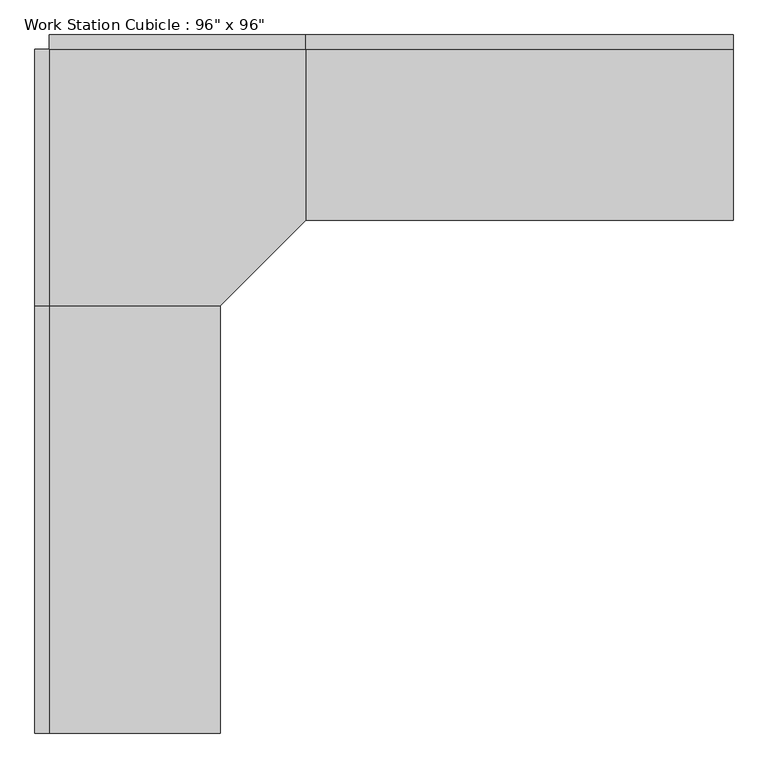
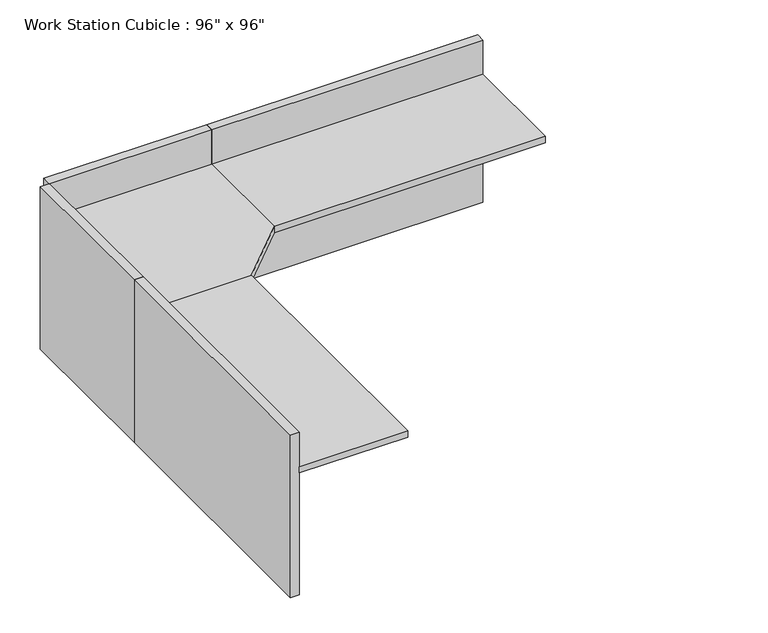
"""IFC4 building model written with IfcOpenShell, lengths in millimetres: furniture geometry."""

from ifc_helpers import new_model, si_unit, frame, origin, origin_with_axes, place, context, project, spatial, polyline, outline, extrude, source, transform, mapped, element, save


def furniture_5c8231d0(model_context):
    return source(origin(), model_context, "Body", "SweptSolid", [
        extrude(outline(polyline([(-80.9317522, -545.8230076), (833.4682478, -545.8230076), (833.4682478, -1155.4230076), (528.6682478, -1460.2230076), (-80.9317522, -1460.2230076), (-80.9317522, -545.8230076)])), frame((0.0, 0.0, 723.9), z_axis=(0.0, 0.0, 1.0), x_axis=(1.0, 0.0, 0.0)), (0.0, 0.0, 1.0), 38.1),
        extrude(outline(polyline([(528.6682478, -2984.2230076), (-80.9317522, -2984.2230076), (-80.9317522, -1460.2230076), (528.6682478, -1460.2230076), (528.6682478, -2984.2230076)])), frame((0.0, 0.0, 723.9), z_axis=(0.0, 0.0, 1.0), x_axis=(1.0, 0.0, 0.0)), (0.0, 0.0, 1.0), 38.1),
        extrude(outline(polyline([(2357.4682478, -1155.4230076), (833.4682478, -1155.4230076), (833.4682478, -545.8230076), (2357.4682478, -545.8230076), (2357.4682478, -1155.4230076)])), frame((0.0, 0.0, 723.9), z_axis=(0.0, 0.0, 1.0), x_axis=(1.0, 0.0, 0.0)), (0.0, 0.0, 1.0), 38.1),
        extrude(outline(polyline([(2357.4682478, -545.8230076), (833.4682478, -545.8230076), (833.4682478, -495.0230076), (2357.4682478, -495.0230076), (2357.4682478, -545.8230076)])), origin_with_axes(), (0.0, 0.0, 1.0), 965.2),
        extrude(outline(polyline([(833.4682478, -545.8230076), (-80.9317522, -545.8230076), (-80.9317522, -495.0230076), (833.4682478, -495.0230076), (833.4682478, -545.8230076)])), origin_with_axes(), (0.0, 0.0, 1.0), 965.2),
        extrude(outline(polyline([(-80.9317522, -1460.2230076), (-131.7317522, -1460.2230076), (-131.7317522, -545.8230076), (-80.9317522, -545.8230076), (-80.9317522, -1460.2230076)])), origin_with_axes(), (0.0, 0.0, 1.0), 965.2),
        extrude(outline(polyline([(-80.9317522, -2984.2230076), (-131.7317522, -2984.2230076), (-131.7317522, -1460.2230076), (-80.9317522, -1460.2230076), (-80.9317522, -2984.2230076)])), origin_with_axes(), (0.0, 0.0, 1.0), 965.2),
    ])


if __name__ == "__main__":
    model = new_model("IFC4")
    model_context = context("Model", 3, world=origin())
    ifc_project = project(units=[si_unit("LENGTHUNIT", "METRE", prefix="MILLI")], contexts=[model_context])
    site = spatial("IfcSite", under=ifc_project)
    building = spatial("IfcBuilding", under=site)
    placement = place(None, origin())
    furniture_shape = furniture_5c8231d0(model_context)
    element("IfcFurniture", 1, ObjectType="Work Station Cubicle : 96\" x 96\"", at=placement, inside=building, context=model_context, shape_type="MappedRepresentation", body=[
        mapped(furniture_shape, transform((0.0, 0.0, 0.0), x_axis=(1.0, 0.0, 0.0), y_axis=(0.0, 1.0, 0.0), z_axis=(0.0, 0.0, 1.0))),
    ])
    save(model, "model.ifc")

# Revit data of these elements
# Type "Work Station Cubicle : 96\" x 96\""
#   Assembly Code = "E2020"
#   Desktop Height = 2' - 6"
#   Desktop1 Width = 2' - 0"
#   Desktop2 Width = 2' - 0"
#   Panel Height = 3' - 2"
#   Panel1 Length = 5' - 0"
#   Panel2 Length = 5' - 0"
#   Cube Panel Material = Textile - Light Gray
#   Work Top Material = Laminate, Ivory, Matte
#   Default Elevation = 0
# Element 1 (IfcFurniture, "Work Station Cubicle : 96\" x 96\"")
#   Materials on its faces: "Textile - Light Gray", "Laminate, Ivory, Matte"
# Materials
#   "Textile - Light Gray": class "Fabric", colour RGB 204 204 204, transparency 0
#   "Laminate, Ivory, Matte": class "Plastic", colour RGB 247 247 239, transparency 0, Description = "Plastic Laminate - Ivory, Matte", Cost = 0
